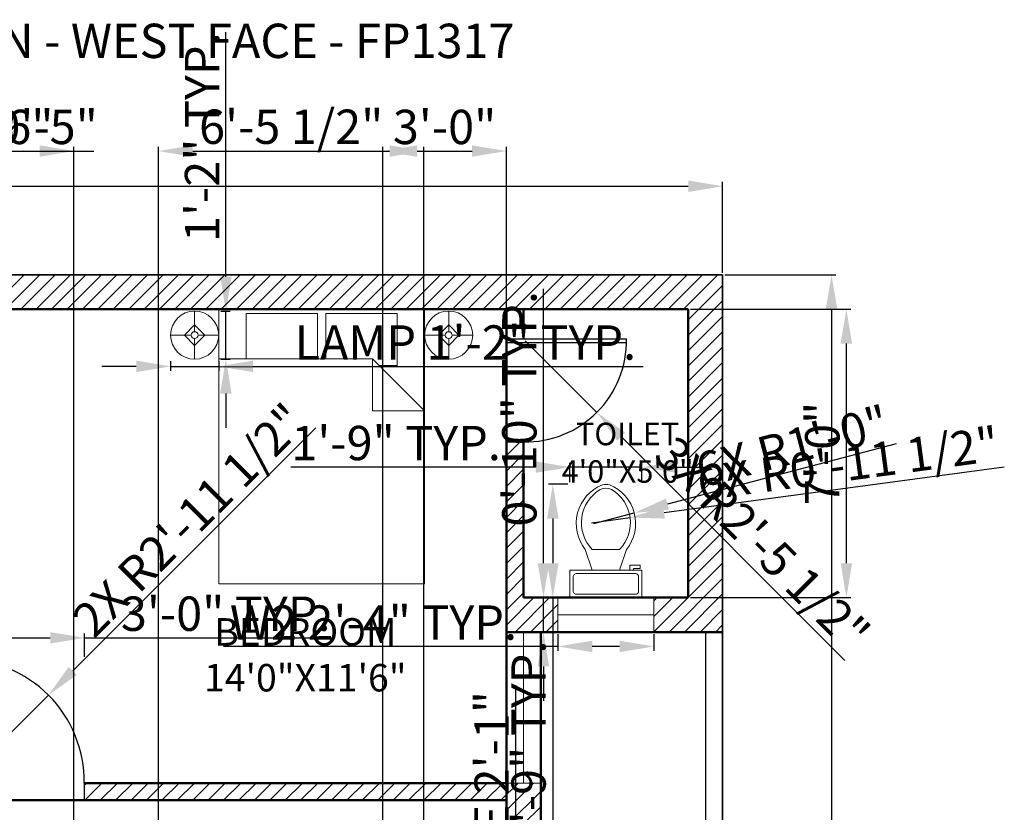
# Model space of a CAD drawing. Units: inches. Extents: x 2206 to 2843, y 1750 to 2489.
# Tile 8 of 8: x 2506 to 2793, y 2238 to 2469. Entities that reach past the tile are written whole.
import ezdxf

# ---------------------------------------------------------------- set-up
doc = ezdxf.new("R2010")
doc.units = ezdxf.units.IN
for name, color, linetype, lineweight in [('A-ANNO-DIMS', 2, 'Continuous', 18), ('A-ANNO-TEXT', 7, 'Continuous', 25), ('A-AREA-IDEN', 7, 'Continuous', 18), ('A-DOOR', 3, 'Continuous', 25), ('A-FLOR-FIXT', 9, 'Continuous', 18), ('A-FURN', 21, 'Continuous', 18), ('A-GLAZ', 4, 'Continuous', 18), ('A-WALL', 7, 'Continuous', 50), ('A-WALL-PATT', 252, 'Continuous', 13), ('C-PROP', 7, 'Continuous', 35), ('L-SITE-WALL', 8, 'Continuous', 25)]:
    doc.layers.add(name, color=color, linetype=linetype, lineweight=lineweight)
doc.styles.get("Standard").update_dxf_attribs({"font": 'arial.ttf'})
doc.dimstyles.new('ISO-25', dxfattribs={"dimtxt": 10, "dimasz": 10, "dimexe": 1.25, "dimexo": 0.625, "dimtad": 1, "dimdec": 1, "dimlunit": 3, "dimtxsty": 'Standard', "dimcen": 2.5, "dimadec": 0, "dimazin": 0, "dimtfac": 1, "dimtdec": 1, "dimtmove": 0, "dimatfit": 3, "dimfxl": 1, "dimarcsym": 0})

# ---------------------------------------------------------------- blocks, each defined once
blk = doc.blocks.new('Bed - Queen')
for p, q in [((0, -80.00003), (0, 0)), ((0, 0), (59.99999, 0)), ((59.99999, 0), (59.99999, -80.00003)), ((7.99999, -1.2), (28.79998, -1.2)), ((7.99999, -14.4), (7.99999, -1.2)), ((28.79998, -1.2), (28.79998, -14.4)), ((31.19999, -1.2), (51.99999, -1.2)), ((31.19999, -14.4), (31.19999, -1.2)), ((51.99999, -1.2), (51.99999, -16.4)), ((0, -14.4), (44.8, -14.4)), ((44.8, -16.8), (0, -16.8)), ((59.99999, -29.6), (44.8, -14.4)), ((44.8, -14.4), (44.8, -29.6)), ((51.99999, -16.4), (46.79936, -16.4)), ((44.8, -29.6), (59.99999, -29.6)), ((59.99999, -80.00003), (0, -80.00003))]:
    blk.add_line(p, q)
blk = doc.blocks.new('Lamp - Table')
for p, q in [((0, 7), (0, 1)), ((0, 3), (-3, 0)), ((3, 0), (0, 3)), ((-1, 0), (-7, 0)), ((-3, 0), (0, -3)), ((0, -3), (3, 0)), ((1, 0), (7, 0)), ((0, -1), (0, -7))]:
    blk.add_line(p, q)
for radius in [7, 1]:
    blk.add_circle((0, 0), radius)
blk = doc.blocks.new('*D14')
at = {"layer": 'A-ANNO-DIMS', "color": 0, "lineweight": -2, "transparency": 16777216}
for p, q in [((2254.58, 2395.52), (2254.58, 2421.96)), ((2710.58, 2395.52), (2710.58, 2421.96)), ((2264.58, 2420.71), (2700.58, 2420.71))]:
    blk.add_line(p, q, dxfattribs=at)
at = {"layer": 'A-ANNO-DIMS', "color": 0, "transparency": 16777216}
for points in [[(2264.58, 2422.38), (2264.58, 2419.04), (2254.58, 2420.71)], [(2700.58, 2422.38), (2700.58, 2419.04), (2710.58, 2420.71)]]:
    blk.add_solid(points, dxfattribs=at)
at = {"layer": 'Defpoints', "color": 0, "transparency": 16777216}
for p in [(2710.58, 2420.71), (2254.58, 2394.9), (2710.58, 2394.9)]:
    blk.add_point(p, dxfattribs=at)
at = {"layer": 'A-ANNO-DIMS', "color": 0, "transparency": 16777216, "insert": (2482.58, 2426.44), "char_height": 10, "attachment_point": 5}
blk.add_mtext("38'", dxfattribs=at)
blk = doc.blocks.new('*D15')
at = {"layer": 'A-ANNO-DIMS', "color": 0, "lineweight": -2, "transparency": 16777216}
for p, q in [((2711.2, 2394.9), (2743.56, 2394.9)), ((2742.31, 2384.9), (2742.31, 1804.9)), ((2711.2, 1794.9), (2743.56, 1794.9))]:
    blk.add_line(p, q, dxfattribs=at)
at = {"layer": 'A-ANNO-DIMS', "color": 0, "transparency": 16777216}
for points in [[(2740.65, 2384.9), (2743.98, 2384.9), (2742.31, 2394.9)], [(2740.65, 1804.9), (2743.98, 1804.9), (2742.31, 1794.9)]]:
    blk.add_solid(points, dxfattribs=at)
at = {"layer": 'Defpoints', "color": 0, "transparency": 16777216}
for p in [(2710.58, 2394.9), (2710.58, 1794.9), (2742.31, 1794.9)]:
    blk.add_point(p, dxfattribs=at)
at = {"layer": 'A-ANNO-DIMS', "color": 0, "transparency": 16777216, "insert": (2736.58, 2094.9), "char_height": 10, "attachment_point": 5, "rotation": 90}
blk.add_mtext("50'", dxfattribs=at)
blk = doc.blocks.new('Toilet - top')
for p, q in [((9.5, -6), (9.5, -2)), ((-10, -8.5), (-8, -8.5)), ((-10, -9.5), (-10, -8.5)), ((-8, -8.5), (-8, -8)), ((-7, -8), (-7, -9.5)), ((-4, -8), (-6, -14)), ((4, -8), (6, -14)), ((-7, -9.5), (-10, -9.5)), ((4, -14), (-4, -14))]:
    blk.add_line(p, q)
blk.add_lwpolyline([(10.5, -8), (10.5, 0), (-10.5, 0), (-10.5, -8)], close=True)
for points in [[(-9.5, -2), (-9.5, -6)], [(8.5, -1), (-8.5, -1)], [(-8.5, -7), (8.5, -7)]]:
    blk.add_lwpolyline(points)
for centre, radius, start, end in [((-8.62, -1.88), 0.884, 81.8699, 188.1301), ((8.62, -1.88), 0.884, 351.8699, 98.1301), ((-8.62, -6.12), 0.884, 171.8699, 278.1301), ((8.62, -6.12), 0.884, 261.8699, 8.1301), ((3.52, -21.58), 12.17, 141.4691, 247.9714), ((4.2, -21.82), 11.33, 136.3677, 238.9468), ((-3.52, -21.58), 12.17, 292.0284, 38.5307), ((-4.2, -21.82), 11.33, 301.053, 43.6321), ((0, -27.88), 4, 245.7318, 294.2682), ((0, -29), 4, 254.8605, 285.1395)]:
    blk.add_arc(centre, radius, start, end)
blk = doc.blocks.new('WIN-28IN')
for p, q in [((10, 28), (0, 28)), ((5, 28), (5, 0)), ((10, 0), (0, 0))]:
    blk.add_line(p, q)
blk = doc.blocks.new('DOOR-SWING-36IN')
for p, q in [((0, 5), (0, 41)), ((1, 0), (1, 41)), ((0, 5), (0, 0)), ((36, 5), (36, 0))]:
    blk.add_line(p, q)
blk.add_arc((0.5, 5.5), 35.5, 359.1931, 90.8069)
blk = doc.blocks.new('*D29')
at = {"layer": 'A-ANNO-DIMS', "color": 0, "lineweight": -2, "transparency": 16777216}
for p, q in [((2549.77, 2369.72), (2549.77, 2367)), ((2563.77, 2369.72), (2563.77, 2367)), ((2539.77, 2368.25), (2529.77, 2368.25)), ((2549.77, 2368.25), (2563.77, 2368.25)), ((2573.77, 2368.25), (2687.46, 2368.25))]:
    blk.add_line(p, q, dxfattribs=at)
at = {"layer": 'A-ANNO-DIMS', "color": 0, "transparency": 16777216}
for points in [[(2539.77, 2369.91), (2539.77, 2366.58), (2549.77, 2368.25)], [(2573.77, 2369.91), (2573.77, 2366.58), (2563.77, 2368.25)]]:
    blk.add_solid(points, dxfattribs=at)
at = {"layer": 'Defpoints', "color": 0, "transparency": 16777216}
for p in [(2549.77, 2370.35), (2563.77, 2370.35), (2563.77, 2368.25)]:
    blk.add_point(p, dxfattribs=at)
at = {"layer": 'A-ANNO-DIMS', "color": 0, "transparency": 16777216, "insert": (2635.61, 2373.9), "char_height": 10, "attachment_point": 5}
blk.add_mtext('LAMP 1\'-2" TYP.', dxfattribs=at)
blk = doc.blocks.new('*D30')
at = {"layer": 'A-ANNO-DIMS', "color": 0, "lineweight": -2, "transparency": 16777216}
for p, q in [((2565.87, 2394.35), (2565.87, 2465.61)), ((2564.4, 2384.35), (2567.12, 2384.35)), ((2565.87, 2370.35), (2565.87, 2384.35)), ((2564.4, 2370.35), (2567.12, 2370.35)), ((2565.87, 2360.35), (2565.87, 2350.35))]:
    blk.add_line(p, q, dxfattribs=at)
at = {"layer": 'A-ANNO-DIMS', "color": 0, "transparency": 16777216}
for points in [[(2564.2, 2394.35), (2567.54, 2394.35), (2565.87, 2384.35)], [(2564.2, 2360.35), (2567.54, 2360.35), (2565.87, 2370.35)]]:
    blk.add_solid(points, dxfattribs=at)
at = {"layer": 'Defpoints', "color": 0, "transparency": 16777216}
for p in [(2563.77, 2384.35), (2565.87, 2384.35), (2563.77, 2370.35)]:
    blk.add_point(p, dxfattribs=at)
at = {"layer": 'A-ANNO-DIMS', "color": 0, "transparency": 16777216, "insert": (2560.22, 2434.98), "char_height": 10, "attachment_point": 5, "rotation": 90}
blk.add_mtext('1\'-2" TYP.', dxfattribs=at)
blk = doc.blocks.new('*D33')
at = {"layer": 'A-ANNO-DIMS', "color": 0, "lineweight": -2, "transparency": 16777216}
for p, q in [((2665.45, 2333.95), (2659.87, 2333.95)), ((2661.12, 2323.95), (2661.12, 2310.9)), ((2665.45, 2300.9), (2659.87, 2300.9)), ((2661.12, 2300.9), (2661.12, 2201.13))]:
    blk.add_line(p, q, dxfattribs=at)
at = {"layer": 'A-ANNO-DIMS', "color": 0, "transparency": 16777216}
for points in [[(2659.46, 2323.95), (2662.79, 2323.95), (2661.12, 2333.95)], [(2659.46, 2310.9), (2662.79, 2310.9), (2661.12, 2300.9)]]:
    blk.add_solid(points, dxfattribs=at)
at = {"layer": 'Defpoints', "color": 0, "transparency": 16777216}
for p in [(2666.08, 2333.95), (2661.12, 2300.9), (2666.08, 2300.9)]:
    blk.add_point(p, dxfattribs=at)
at = {"layer": 'A-ANNO-DIMS', "color": 0, "transparency": 16777216, "insert": (2655.33, 2246.01), "char_height": 10, "attachment_point": 5, "rotation": 90}
blk.add_mtext('WC 2\'-9" TYP.', dxfattribs=at)
blk = doc.blocks.new('*D34')
at = {"layer": 'A-ANNO-DIMS', "color": 0, "lineweight": -2, "transparency": 16777216}
for p, q in [((2656.08, 2338.9), (2584.82, 2338.9)), ((2666.08, 2334.57), (2666.08, 2340.15)), ((2687.08, 2338.9), (2666.08, 2338.9)), ((2687.08, 2334.57), (2687.08, 2340.15)), ((2697.08, 2338.9), (2707.08, 2338.9))]:
    blk.add_line(p, q, dxfattribs=at)
at = {"layer": 'A-ANNO-DIMS', "color": 0, "transparency": 16777216}
for points in [[(2656.08, 2340.57), (2656.08, 2337.24), (2666.08, 2338.9)], [(2697.08, 2340.57), (2697.08, 2337.24), (2687.08, 2338.9)]]:
    blk.add_solid(points, dxfattribs=at)
at = {"layer": 'Defpoints', "color": 0, "transparency": 16777216}
for p in [(2666.08, 2338.9), (2666.08, 2333.95), (2687.08, 2333.95)]:
    blk.add_point(p, dxfattribs=at)
at = {"layer": 'A-ANNO-DIMS', "color": 0, "transparency": 16777216, "insert": (2615.45, 2344.63), "char_height": 10, "attachment_point": 5}
blk.add_mtext('1\'-9" TYP.', dxfattribs=at)
blk = doc.blocks.new('*D37')
at = {"layer": 'A-ANNO-DIMS', "color": 0, "lineweight": -2, "transparency": 16777216}
for p, q in [((2662.58, 2290.27), (2662.58, 2285.45)), ((2690.58, 2290.27), (2690.58, 2285.45)), ((2662.58, 2286.7), (2565.13, 2286.7)), ((2680.58, 2286.7), (2672.58, 2286.7))]:
    blk.add_line(p, q, dxfattribs=at)
at = {"layer": 'A-ANNO-DIMS', "color": 0, "transparency": 16777216}
for points in [[(2672.58, 2288.37), (2672.58, 2285.03), (2662.58, 2286.7)], [(2680.58, 2288.37), (2680.58, 2285.03), (2690.58, 2286.7)]]:
    blk.add_solid(points, dxfattribs=at)
at = {"layer": 'Defpoints', "color": 0, "transparency": 16777216}
for p in [(2662.58, 2290.9), (2690.58, 2290.9), (2662.58, 2286.7)]:
    blk.add_point(p, dxfattribs=at)
at = {"layer": 'A-ANNO-DIMS', "color": 0, "transparency": 16777216, "insert": (2608.85, 2292.35), "char_height": 10, "attachment_point": 5}
blk.add_mtext('W2 2\'-4" TYP.', dxfattribs=at)
blk = doc.blocks.new('*D38')
at = {"layer": 'A-ANNO-DIMS', "color": 0, "lineweight": -2, "transparency": 16777216}
for p, q in [((2658.38, 2310.9), (2658.38, 2390.87)), ((2661.95, 2300.9), (2657.13, 2300.9)), ((2658.38, 2290.9), (2658.38, 2300.9)), ((2661.95, 2290.9), (2657.13, 2290.9)), ((2658.38, 2280.9), (2658.38, 2270.9))]:
    blk.add_line(p, q, dxfattribs=at)
at = {"layer": 'A-ANNO-DIMS', "color": 0, "transparency": 16777216}
for points in [[(2656.71, 2310.9), (2660.05, 2310.9), (2658.38, 2300.9)], [(2656.71, 2280.9), (2660.05, 2280.9), (2658.38, 2290.9)]]:
    blk.add_solid(points, dxfattribs=at)
at = {"layer": 'Defpoints', "color": 0, "transparency": 16777216}
for p in [(2658.38, 2300.9), (2662.58, 2300.9), (2662.58, 2290.9)]:
    blk.add_point(p, dxfattribs=at)
at = {"layer": 'A-ANNO-DIMS', "color": 0, "transparency": 16777216, "insert": (2652.65, 2355.89), "char_height": 10, "attachment_point": 5, "rotation": 90}
blk.add_mtext('0\'-10" TYP.', dxfattribs=at)
blk = doc.blocks.new('*D42')
at = {"layer": 'A-ANNO-DIMS', "color": 0, "lineweight": -2, "transparency": 16777216}
for p, q in [((2488.58, 2283.66), (2488.58, 2290.45)), ((2498.58, 2289.2), (2514.71, 2289.2)), ((2524.71, 2283.66), (2524.71, 2290.45)), ((2524.71, 2289.2), (2596.91, 2289.2))]:
    blk.add_line(p, q, dxfattribs=at)
at = {"layer": 'A-ANNO-DIMS', "color": 0, "transparency": 16777216}
for points in [[(2498.58, 2290.87), (2498.58, 2287.54), (2488.58, 2289.2)], [(2514.71, 2290.87), (2514.71, 2287.54), (2524.71, 2289.2)]]:
    blk.add_solid(points, dxfattribs=at)
at = {"layer": 'Defpoints', "color": 0, "transparency": 16777216}
for p in [(2524.71, 2289.2), (2488.58, 2283.03), (2524.71, 2283.03)]:
    blk.add_point(p, dxfattribs=at)
at = {"layer": 'A-ANNO-DIMS', "color": 0, "transparency": 16777216, "insert": (2565.81, 2294.94), "char_height": 10, "attachment_point": 5}
blk.add_mtext('3\'-0" TYP.', dxfattribs=at)
blk = doc.blocks.new('*D53')
at = {"layer": 'A-ANNO-DIMS', "color": 0, "lineweight": -2, "transparency": 16777216}
for p, q in [((2650.37, 2184.58), (2650.37, 2275.46)), ((2647.27, 2184.58), (2651.62, 2184.58)), ((2650.37, 2169.75), (2650.37, 2174.58)), ((2647.27, 2159.75), (2651.62, 2159.75))]:
    blk.add_line(p, q, dxfattribs=at)
at = {"layer": 'A-ANNO-DIMS', "color": 0, "transparency": 16777216}
for points in [[(2648.71, 2174.58), (2652.04, 2174.58), (2650.37, 2184.58)], [(2648.71, 2169.75), (2652.04, 2169.75), (2650.37, 2159.75)]]:
    blk.add_solid(points, dxfattribs=at)
at = {"layer": 'Defpoints', "color": 0, "transparency": 16777216}
for p in [(2646.65, 2184.58), (2650.37, 2184.58), (2646.65, 2159.75)]:
    blk.add_point(p, dxfattribs=at)
at = {"layer": 'A-ANNO-DIMS', "color": 0, "transparency": 16777216, "insert": (2644.58, 2235.02), "char_height": 10, "attachment_point": 5, "rotation": 90}
blk.add_mtext('RANGE 2\'-1"', dxfattribs=at)
blk = doc.blocks.new('*D61')
at = {"layer": 'A-ANNO-DIMS', "color": 0, "lineweight": -2, "transparency": 16777216}
for p, q in [((2479.58, 2100.52), (2479.58, 2432.2)), ((2489.58, 2430.95), (2511.58, 2430.95)), ((2521.58, 2100.52), (2521.58, 2432.2))]:
    blk.add_line(p, q, dxfattribs=at)
at = {"layer": 'A-ANNO-DIMS', "color": 0, "transparency": 16777216}
for points in [[(2489.58, 2432.62), (2489.58, 2429.28), (2479.58, 2430.95)], [(2511.58, 2432.62), (2511.58, 2429.28), (2521.58, 2430.95)]]:
    blk.add_solid(points, dxfattribs=at)
at = {"layer": 'Defpoints', "color": 0, "transparency": 16777216}
for p in [(2521.58, 2430.95), (2479.58, 2099.9), (2521.58, 2099.9)]:
    blk.add_point(p, dxfattribs=at)
at = {"layer": 'A-ANNO-DIMS', "color": 0, "transparency": 16777216, "insert": (2500.58, 2436.68), "char_height": 10, "attachment_point": 5}
blk.add_mtext('3\'-6"', dxfattribs=at)
blk = doc.blocks.new('*D63')
at = {"layer": 'A-ANNO-DIMS', "color": 0, "lineweight": -2, "transparency": 16777216}
for p, q in [((2647.58, 2246.27), (2647.58, 1757.6)), ((2657.58, 2246.27), (2657.58, 1757.6)), ((2637.58, 1758.85), (2627.58, 1758.85)), ((2647.58, 1758.85), (2657.58, 1758.85)), ((2667.58, 1758.85), (2713.18, 1758.85))]:
    blk.add_line(p, q, dxfattribs=at)
at = {"layer": 'A-ANNO-DIMS', "color": 0, "transparency": 16777216}
for points in [[(2637.58, 1760.52), (2637.58, 1757.18), (2647.58, 1758.85)], [(2667.58, 1760.52), (2667.58, 1757.18), (2657.58, 1758.85)]]:
    blk.add_solid(points, dxfattribs=at)
at = {"layer": 'Defpoints', "color": 0, "transparency": 16777216}
for p in [(2647.58, 2246.9), (2657.58, 2246.9), (2657.58, 1758.85)]:
    blk.add_point(p, dxfattribs=at)
at = {"layer": 'A-ANNO-DIMS', "color": 0, "transparency": 16777216, "insert": (2695.38, 1764.58), "char_height": 10, "attachment_point": 5}
blk.add_mtext('0\'-10"', dxfattribs=at)
blk = doc.blocks.new('*D64')
at = {"layer": 'A-ANNO-DIMS', "color": 0, "lineweight": -2, "transparency": 16777216}
for p, q in [((2701.2, 2384.9), (2747.88, 2384.9)), ((2746.63, 2310.9), (2746.63, 2374.9)), ((2701.2, 2300.9), (2747.88, 2300.9))]:
    blk.add_line(p, q, dxfattribs=at)
at = {"layer": 'A-ANNO-DIMS', "color": 0, "transparency": 16777216}
for points in [[(2744.96, 2374.9), (2748.3, 2374.9), (2746.63, 2384.9)], [(2744.96, 2310.9), (2748.3, 2310.9), (2746.63, 2300.9)]]:
    blk.add_solid(points, dxfattribs=at)
at = {"layer": 'Defpoints', "color": 0, "transparency": 16777216}
for p in [(2700.58, 2384.9), (2746.63, 2384.9), (2700.58, 2300.9)]:
    blk.add_point(p, dxfattribs=at)
at = {"layer": 'A-ANNO-DIMS', "color": 0, "transparency": 16777216, "insert": (2740.9, 2342.9), "char_height": 10, "attachment_point": 5, "rotation": 90}
blk.add_mtext('7\'-0"', dxfattribs=at)
blk = doc.blocks.new('*D65')
at = {"layer": 'A-ANNO-DIMS', "color": 0, "lineweight": -2, "transparency": 16777216}
for p, q in [((2464.58, 2430.95), (2454.58, 2430.95)), ((2474.58, 2385.52), (2474.58, 2432.2)), ((2474.58, 2430.95), (2479.58, 2430.95)), ((2479.58, 2385.52), (2479.58, 2432.2)), ((2489.58, 2430.95), (2527.41, 2430.95))]:
    blk.add_line(p, q, dxfattribs=at)
at = {"layer": 'A-ANNO-DIMS', "color": 0, "transparency": 16777216}
for points in [[(2464.58, 2432.62), (2464.58, 2429.28), (2474.58, 2430.95)], [(2489.58, 2432.62), (2489.58, 2429.28), (2479.58, 2430.95)]]:
    blk.add_solid(points, dxfattribs=at)
at = {"layer": 'Defpoints', "color": 0, "transparency": 16777216}
for p in [(2479.58, 2430.95), (2474.58, 2384.9), (2479.58, 2384.9)]:
    blk.add_point(p, dxfattribs=at)
at = {"layer": 'A-ANNO-DIMS', "color": 0, "transparency": 16777216, "insert": (2513.5, 2436.68), "char_height": 10, "attachment_point": 5}
blk.add_mtext('0\'-5"', dxfattribs=at)
blk = doc.blocks.new('*D74')
at = {"layer": 'A-ANNO-DIMS', "color": 0, "lineweight": -2, "transparency": 16777216}
for p, q in [((2611.58, 1856.52), (2611.58, 2432.2)), ((2621.58, 2430.95), (2637.58, 2430.95)), ((2647.58, 1856.52), (2647.58, 2432.2))]:
    blk.add_line(p, q, dxfattribs=at)
at = {"layer": 'A-ANNO-DIMS', "color": 0, "transparency": 16777216}
for points in [[(2621.58, 2432.62), (2621.58, 2429.28), (2611.58, 2430.95)], [(2637.58, 2432.62), (2637.58, 2429.28), (2647.58, 2430.95)]]:
    blk.add_solid(points, dxfattribs=at)
at = {"layer": 'Defpoints', "color": 0, "transparency": 16777216}
for p in [(2647.58, 2430.95), (2611.58, 1855.9), (2647.58, 1855.9)]:
    blk.add_point(p, dxfattribs=at)
at = {"layer": 'A-ANNO-DIMS', "color": 0, "transparency": 16777216, "insert": (2629.58, 2436.68), "char_height": 10, "attachment_point": 5}
blk.add_mtext('3\'-0"', dxfattribs=at)
blk = doc.blocks.new('*D79')
at = {"layer": 'A-ANNO-DIMS', "color": 0, "lineweight": -2, "transparency": 16777216}
for p, q in [((2546.21, 2129.52), (2546.21, 2432.2)), ((2556.21, 2430.95), (2613.58, 2430.95)), ((2623.58, 2129.52), (2623.58, 2432.2))]:
    blk.add_line(p, q, dxfattribs=at)
at = {"layer": 'A-ANNO-DIMS', "color": 0, "transparency": 16777216}
for points in [[(2556.21, 2432.62), (2556.21, 2429.28), (2546.21, 2430.95)], [(2613.58, 2432.62), (2613.58, 2429.28), (2623.58, 2430.95)]]:
    blk.add_solid(points, dxfattribs=at)
at = {"layer": 'Defpoints', "color": 0, "transparency": 16777216}
for p in [(2623.58, 2430.95), (2546.21, 2128.9), (2623.58, 2128.9)]:
    blk.add_point(p, dxfattribs=at)
at = {"layer": 'A-ANNO-DIMS', "color": 0, "transparency": 16777216, "insert": (2584.9, 2436.74), "char_height": 10, "attachment_point": 5}
blk.add_mtext('6\'-5 1/2"', dxfattribs=at)
blk = doc.blocks.new('*D83')
at = {"layer": 'A-ANNO-DIMS', "color": 0, "lineweight": -2, "transparency": 16777216}
for p, q in [((2592.06, 2350.38), (2521.26, 2279.57)), ((2489.08, 2247.4), (2514.18, 2272.5))]:
    blk.add_line(p, q, dxfattribs=at)
at = {"layer": 'A-ANNO-DIMS', "color": 0, "transparency": 16777216}
blk.add_solid([(2520.08, 2280.75), (2522.43, 2278.4), (2514.18, 2272.5)], dxfattribs=at)
at = {"layer": 'Defpoints', "color": 0, "transparency": 16777216}
for p in [(2514.18, 2272.5), (2489.08, 2247.4)]:
    blk.add_point(p, dxfattribs=at)
at = {"layer": 'A-ANNO-DIMS', "color": 0, "transparency": 16777216, "insert": (2556.1, 2322.61), "char_height": 10, "attachment_point": 5, "rotation": 44.9995}
blk.add_mtext('2X R2\'-11 1/2"', dxfattribs=at)
blk = doc.blocks.new('*D84')
at = {"layer": 'A-ANNO-DIMS', "color": 0, "lineweight": -2, "transparency": 16777216}
for p, q in [((2653.08, 2375.73), (2673.94, 2354.86)), ((2746.2, 2282.61), (2681.01, 2347.79))]:
    blk.add_line(p, q, dxfattribs=at)
at = {"layer": 'A-ANNO-DIMS', "color": 0, "transparency": 16777216}
blk.add_solid([(2682.19, 2348.97), (2679.83, 2346.62), (2673.94, 2354.86)], dxfattribs=at)
at = {"layer": 'Defpoints', "color": 0, "transparency": 16777216}
for p in [(2653.08, 2375.73), (2673.94, 2354.86)]:
    blk.add_point(p, dxfattribs=at)
at = {"layer": 'A-ANNO-DIMS', "color": 0, "transparency": 16777216, "insert": (2721.24, 2315.77), "char_height": 10, "attachment_point": 5, "rotation": 314.9998}
blk.add_mtext('3X R2\'-5 1/2"', dxfattribs=at)
blk = doc.blocks.new('*D85')
at = {"layer": 'A-ANNO-DIMS', "color": 0, "lineweight": -2, "transparency": 16777216}
for p, q in [((2761.17, 2345.69), (2694.5, 2328.13)), ((2673.06, 2322.48), (2684.83, 2325.58))]:
    blk.add_line(p, q, dxfattribs=at)
at = {"layer": 'A-ANNO-DIMS', "color": 0, "transparency": 16777216}
blk.add_solid([(2694.07, 2329.74), (2694.92, 2326.51), (2684.83, 2325.58)], dxfattribs=at)
at = {"layer": 'Defpoints', "color": 0, "transparency": 16777216}
for p in [(2684.83, 2325.58), (2673.06, 2322.48)]:
    blk.add_point(p, dxfattribs=at)
at = {"layer": 'A-ANNO-DIMS', "color": 0, "transparency": 16777216, "insert": (2731.21, 2343.72), "char_height": 10, "attachment_point": 5, "rotation": 14.7571}
blk.add_mtext('6X R1\'-0"', dxfattribs=at)
blk = doc.blocks.new('*D86')
at = {"layer": 'A-ANNO-DIMS', "color": 0, "lineweight": -2, "transparency": 16777216}
for p, q in [((2792.64, 2338.94), (2693.52, 2325.57)), ((2672.38, 2322.72), (2683.61, 2324.23))]:
    blk.add_line(p, q, dxfattribs=at)
at = {"layer": 'A-ANNO-DIMS', "color": 0, "transparency": 16777216}
blk.add_solid([(2693.29, 2327.22), (2693.74, 2323.92), (2683.61, 2324.23)], dxfattribs=at)
at = {"layer": 'Defpoints', "color": 0, "transparency": 16777216}
for p in [(2683.61, 2324.23), (2672.38, 2322.72)]:
    blk.add_point(p, dxfattribs=at)
at = {"layer": 'A-ANNO-DIMS', "color": 0, "transparency": 16777216, "insert": (2747.26, 2338.67), "char_height": 10, "attachment_point": 5, "rotation": 7.6826}
blk.add_mtext('6X R0\'-11 1/2"', dxfattribs=at)

msp = doc.modelspace()

# ---------------------------------------------------------------- hatches: boundary and pattern name
at = {"layer": 'A-WALL-PATT'}
h = msp.add_hatch(dxfattribs=at)
h.set_pattern_fill('ANSI31', color=256)
h.paths.add_polyline_path([(2710.58, 2394.9), (2296.58, 2394.9), (2296.58, 2335.9), (2306.58, 2335.9), (2306.58, 2384.9), (2479.58, 2384.9), (2652.58, 2384.9), (2700.58, 2384.9), (2700.58, 2300.9), (2690.58, 2300.9), (2690.58, 2290.9), (2710.58, 2290.9)])
h.paths.add_polyline_path([(2306.58, 2295.9), (2296.58, 2295.9), (2296.58, 2225.9), (2306.58, 2225.9), (2306.58, 2241.9)])
h.paths.add_polyline_path([(2306.58, 2111.9), (2306.58, 2132.9), (2296.58, 2132.9), (2296.58, 2071.9), (2306.58, 2071.9)])
h.paths.add_polyline_path([(2306.58, 2197.9), (2296.58, 2197.9), (2296.58, 2160.9), (2306.58, 2160.9), (2306.58, 2176.9)])
h.paths.add_polyline_path([(2370.58, 1991.9), (2306.58, 1991.9), (2306.58, 2031.9), (2296.58, 2031.9), (2296.58, 1981.9), (2370.58, 1981.9)])
h.paths.add_polyline_path([(2479.58, 2066.9), (2474.58, 2066.9), (2474.58, 1991.9), (2410.58, 1991.9), (2410.58, 1981.9), (2479.58, 1981.9)])
h.paths.add_polyline_path([(2539.58, 1943.9), (2479.58, 1943.9), (2479.58, 1944.9), (2469.58, 1944.9), (2469.58, 1933.9), (2539.58, 1933.9)])
h.paths.add_polyline_path([(2657.58, 1997.9), (2647.58, 1997.9), (2647.58, 1943.9), (2647.58, 1918.9), (2657.58, 1918.9)])
h.paths.add_polyline_path([(2647.58, 1943.9), (2587.58, 1943.9), (2587.58, 1933.9), (2647.58, 1933.9)])
h.paths.add_polyline_path([(2657.58, 2158.4), (2647.58, 2158.4), (2647.58, 2104.9), (2647.58, 2045.9), (2657.58, 2045.9)])
h.paths.add_polyline_path([(2657.58, 2204.89), (2647.58, 2204.89), (2647.58, 2188.4), (2657.58, 2188.4)])
h.paths.add_polyline_path([(2657.58, 2246.9), (2647.58, 2246.9), (2647.58, 2234.9), (2657.58, 2234.9)])
h.paths.add_polyline_path([(2662.58, 2300.9), (2652.58, 2300.9), (2652.58, 2346.22), (2647.58, 2346.22), (2647.58, 2290.9), (2662.58, 2290.9)])
h.paths.add_polyline_path([(2647.58, 2246.9), (2524.58, 2246.9), (2524.58, 2241.9), (2647.58, 2241.9)])
h.paths.add_polyline_path([(2351.58, 2246.9), (2306.58, 2246.9), (2306.58, 2241.9), (2351.58, 2241.9)])
h.paths.add_polyline_path([(2429.58, 2246.9), (2381.58, 2246.9), (2381.58, 2241.9), (2390.58, 2241.9), (2390.58, 2181.9), (2306.58, 2181.9), (2306.58, 2176.9), (2390.58, 2176.9), (2390.58, 2116.9), (2381.58, 2116.9), (2381.58, 2111.9), (2474.58, 2111.9), (2474.58, 2102.9), (2479.58, 2102.9), (2479.58, 2104.9), (2479.58, 2116.9), (2395.58, 2116.9), (2395.58, 2176.9), (2395.58, 2241.9), (2429.58, 2241.9)])
h.paths.add_polyline_path([(2479.58, 2384.9), (2474.58, 2384.9), (2474.58, 2246.9), (2465.58, 2246.9), (2465.58, 2241.9), (2479.58, 2241.9), (2488.58, 2241.9), (2488.58, 2246.9), (2479.58, 2246.9)])
h.paths.add_polyline_path([(2657.58, 1870.9), (2647.58, 1870.9), (2647.58, 1855.9), (2511.58, 1855.9), (2511.58, 1845.9), (2657.58, 1845.9)])

# ---------------------------------------------------------------- linework, layer by layer
at = {"layer": 'A-DOOR'}
for p, q in [((2647.58, 2376.23), (2682.58, 2376.23)), ((2647.58, 2375.23), (2682.58, 2375.23)), ((2653.08, 2346.22), (2647.58, 2346.22))]:
    msp.add_line(p, q, dxfattribs=at)
msp.add_arc((2653.08, 2375.73), 29.5, 269.029, 0.971, dxfattribs=at)
at = {"layer": 'A-GLAZ'}
for p, q in [((2652.58, 2290.9), (2652.58, 2246.9)), ((2657.58, 2246.9), (2647.58, 2246.9))]:
    msp.add_line(p, q, dxfattribs=at)
at = {"layer": 'A-WALL'}
for p, q in [((2479.58, 2384.9), (2652.58, 2384.9)), ((2647.58, 2384.9), (2647.58, 2246.9)), ((2652.58, 2384.9), (2700.58, 2384.9)), ((2652.58, 2384.9), (2652.58, 2376.23)), ((2700.58, 2384.9), (2700.58, 2300.9)), ((2652.58, 2346.23), (2652.58, 2300.9)), ((2652.58, 2300.9), (2700.58, 2300.9)), ((2647.58, 2290.9), (2710.58, 2290.9)), ((2657.58, 2290.9), (2657.58, 1845.9)), ((2524.58, 2246.9), (2647.58, 2246.9)), ((2647.58, 2246.9), (2647.58, 2234.9)), ((2479.58, 2241.9), (2647.58, 2241.9))]:
    msp.add_line(p, q, dxfattribs=at)
at = {"layer": 'C-PROP'}
for p, q in [((2254.58, 2394.9), (2710.58, 2394.9)), ((2710.58, 2394.9), (2710.58, 1794.9))]:
    msp.add_line(p, q, dxfattribs=at)
at = {"layer": 'L-SITE-WALL'}
msp.add_line((2705.58, 2290.9), (2705.58, 1799.9), dxfattribs=at)

# ---------------------------------------------------------------- block references
at = {"layer": 'A-DOOR'}
msp.add_blockref('DOOR-SWING-36IN', (2488.58, 2241.9), dxfattribs=at)
at = {"layer": 'A-FLOR-FIXT', "rotation": 180}
msp.add_blockref('Toilet - top', (2676.58, 2300.9), dxfattribs=at)
at = {"layer": 'A-FURN'}
for name, p in [('Lamp - Table', (2556.77, 2377.35)), ('Bed - Queen', (2563.77, 2384.89))]:
    msp.add_blockref(name, p, dxfattribs=at)
at = {"layer": 'A-FURN', "xscale": -1}
msp.add_blockref('Lamp - Table', (2630.77, 2377.35), dxfattribs=at)
at = {"layer": 'A-GLAZ', "rotation": 90.00000000000284}
msp.add_blockref('WIN-28IN', (2690.58, 2290.9), dxfattribs=at)

# ---------------------------------------------------------------- texts
at = {"layer": 'A-ANNO-TEXT', "insert": (2305.82, 2468.04), "char_height": 10, "attachment_point": 1}
msp.add_mtext_dynamic_manual_height_columns('{\\fArial|b1|i0|c0|p34;38X50 (1900 SQFT) HOUSE PLAN - WEST FACE - FP1317}', width=488.3638, gutter_width=12.5, heights=[0], dxfattribs=at)
at = {"layer": 'A-AREA-IDEN', "attachment_point": 1}
for s, width, gutter_width, insert, char_height in [('\\pxqc;TOILET\\P4\'0"X5\'0"', 75.366, 10.24, (2645.21, 2351.84), 6.5536), ('\\pxqc;BEDROOM\\P14\'0"X11\'6"', 91.9993, 12.5, (2543, 2294.93), 8)]:
    msp.add_mtext_dynamic_manual_height_columns(s, width=width, gutter_width=gutter_width, heights=[0], dxfattribs=dict(at, insert=insert, char_height=char_height))

# ---------------------------------------------------------------- dimensions: what is measured, and where the dimension line sits
at = {"layer": 'A-ANNO-DIMS'}
for base, p1, p2, angle, text, picture, middle in [((2565.87, 2384.35), (2563.77, 2370.35), (2563.77, 2384.35), 90, '<> TYP.', '*D30', (2560.22, 2434.98)), ((2658.38, 2300.9), (2662.58, 2290.9), (2662.58, 2300.9), 90, '<> TYP.', '*D38', (2652.65, 2355.89)), ((2666.08, 2338.9), (2687.08, 2333.95), (2666.08, 2333.95), 180, '<> TYP.', '*D34', (2615.45, 2344.63)), ((2661.1228, 2300.8992), (2666.0797, 2333.9455), (2666.0797, 2300.8992), 270, 'WC <> TYP.', '*D33', (2655.3273, 2246.0143)), ((2662.58, 2286.7), (2690.58, 2290.9), (2662.58, 2290.9), 180, 'W2 <> TYP.', '*D37', (2608.85, 2292.35)), ((2650.37, 2184.58), (2646.65, 2159.75), (2646.65, 2184.58), 90, 'RANGE <>', '*D53', (2644.58, 2235.02))]:
    dim = msp.add_linear_dim(base=base, p1=p1, p2=p2, angle=angle, text=text, dimstyle='ISO-25', override={"dimdec": 1, "dimlfac": 1, "dimrnd": 0, "dimzin": 1, "dimdsep": 46, "dimlunit": 4, "dimfrac": 2}, dxfattribs=at)
    dim.commit()
    dim.dimension.update_dxf_attribs({"geometry": picture, "text_midpoint": middle})
for base, p1, p2, override, picture, middle in [((2623.58, 2430.95), (2546.21, 2128.9), (2623.58, 2128.9), {"dimdec": 1, "dimlfac": 1, "dimrnd": 0, "dimzin": 1, "dimdsep": 46, "dimlunit": 4, "dimfrac": 2}, '*D79', (2584.9, 2436.74)), ((2479.58, 2430.95), (2474.58, 2384.9), (2479.58, 2384.9), {"dimdec": 1, "dimlfac": 1, "dimrnd": 0, "dimzin": 1, "dimdsep": 46, "dimlunit": 4, "dimfrac": 2}, '*D65', (2513.5, 2436.68)), ((2521.58, 2430.95), (2479.58, 2099.9), (2521.58, 2099.9), {"dimdec": 1, "dimlfac": 1, "dimrnd": 0, "dimzin": 1, "dimdsep": 46, "dimlunit": 4, "dimfrac": 2}, '*D61', (2500.58, 2436.68)), ((2647.58, 2430.95), (2611.58, 1855.9), (2647.58, 1855.9), {"dimdec": 1, "dimlfac": 1, "dimrnd": 0, "dimzin": 1, "dimdsep": 46, "dimlunit": 4, "dimfrac": 2}, '*D74', (2629.58, 2436.68)), ((2710.58, 2420.71), (2254.58, 2394.9), (2710.58, 2394.9), {"dimclrd": 0, "dimclre": 0, "dimclrt": 0}, '*D14', (2482.58, 2426.44)), ((2657.58, 1758.85), (2647.58, 2246.9), (2657.58, 2246.9), {"dimdec": 1, "dimlfac": 1, "dimrnd": 0, "dimzin": 1, "dimdsep": 46, "dimlunit": 4, "dimfrac": 2}, '*D63', (2695.38, 1764.58))]:
    dim = msp.add_linear_dim(base=base, p1=p1, p2=p2, dimstyle='ISO-25', override=override, dxfattribs=at)
    dim.commit()
    dim.dimension.update_dxf_attribs({"geometry": picture, "text_midpoint": middle})
for base, p1, p2, text, picture, middle in [((2563.77, 2368.25), (2549.77, 2370.35), (2563.77, 2370.35), 'LAMP <> TYP.', '*D29', (2635.61, 2373.9)), ((2524.71, 2289.2), (2488.58, 2283.03), (2524.71, 2283.03), '<> TYP.', '*D42', (2565.81, 2294.94))]:
    dim = msp.add_linear_dim(base=base, p1=p1, p2=p2, text=text, dimstyle='ISO-25', override={"dimdec": 1, "dimlfac": 1, "dimrnd": 0, "dimzin": 1, "dimdsep": 46, "dimlunit": 4, "dimfrac": 2}, dxfattribs=at)
    dim.commit()
    dim.dimension.update_dxf_attribs({"geometry": picture, "text_midpoint": middle})
for base, p1, p2, override, picture, middle in [((2742.31, 1794.9), (2710.58, 2394.9), (2710.58, 1794.9), {"dimclrd": 0, "dimclre": 0, "dimclrt": 0}, '*D15', (2736.58, 2094.9)), ((2746.63, 2384.9), (2700.58, 2300.9), (2700.58, 2384.9), {"dimdec": 1, "dimlfac": 1, "dimrnd": 0, "dimzin": 1, "dimdsep": 46, "dimlunit": 4, "dimfrac": 2}, '*D64', (2740.9, 2342.9))]:
    dim = msp.add_linear_dim(base=base, p1=p1, p2=p2, angle=90, dimstyle='ISO-25', override=override, dxfattribs=at)
    dim.commit()
    dim.dimension.update_dxf_attribs({"geometry": picture, "text_midpoint": middle})
for center, mpoint, text, picture, middle in [((2653.08, 2375.73), (2673.94, 2354.86), '3X <>', '*D84', (2721.24, 2315.77)), ((2672.38, 2322.72), (2683.61, 2324.23), '6X <>', '*D86', (2747.26, 2338.67)), ((2673.06, 2322.48), (2684.83, 2325.58), '6X <>', '*D85', (2731.21, 2343.72)), ((2489.08, 2247.4), (2514.18, 2272.5), '2X <>', '*D83', (2556.1, 2322.61))]:
    dim = msp.add_radius_dim(center=center, mpoint=mpoint, text=text, dimstyle='ISO-25', override={"dimdec": 1, "dimlfac": 1, "dimrnd": 0, "dimzin": 1, "dimdsep": 46, "dimlunit": 4, "dimfrac": 2}, dxfattribs=at)
    dim.commit()
    dim.dimension.update_dxf_attribs({"geometry": picture, "text_midpoint": middle})

doc.saveas('drawing.dxf')
